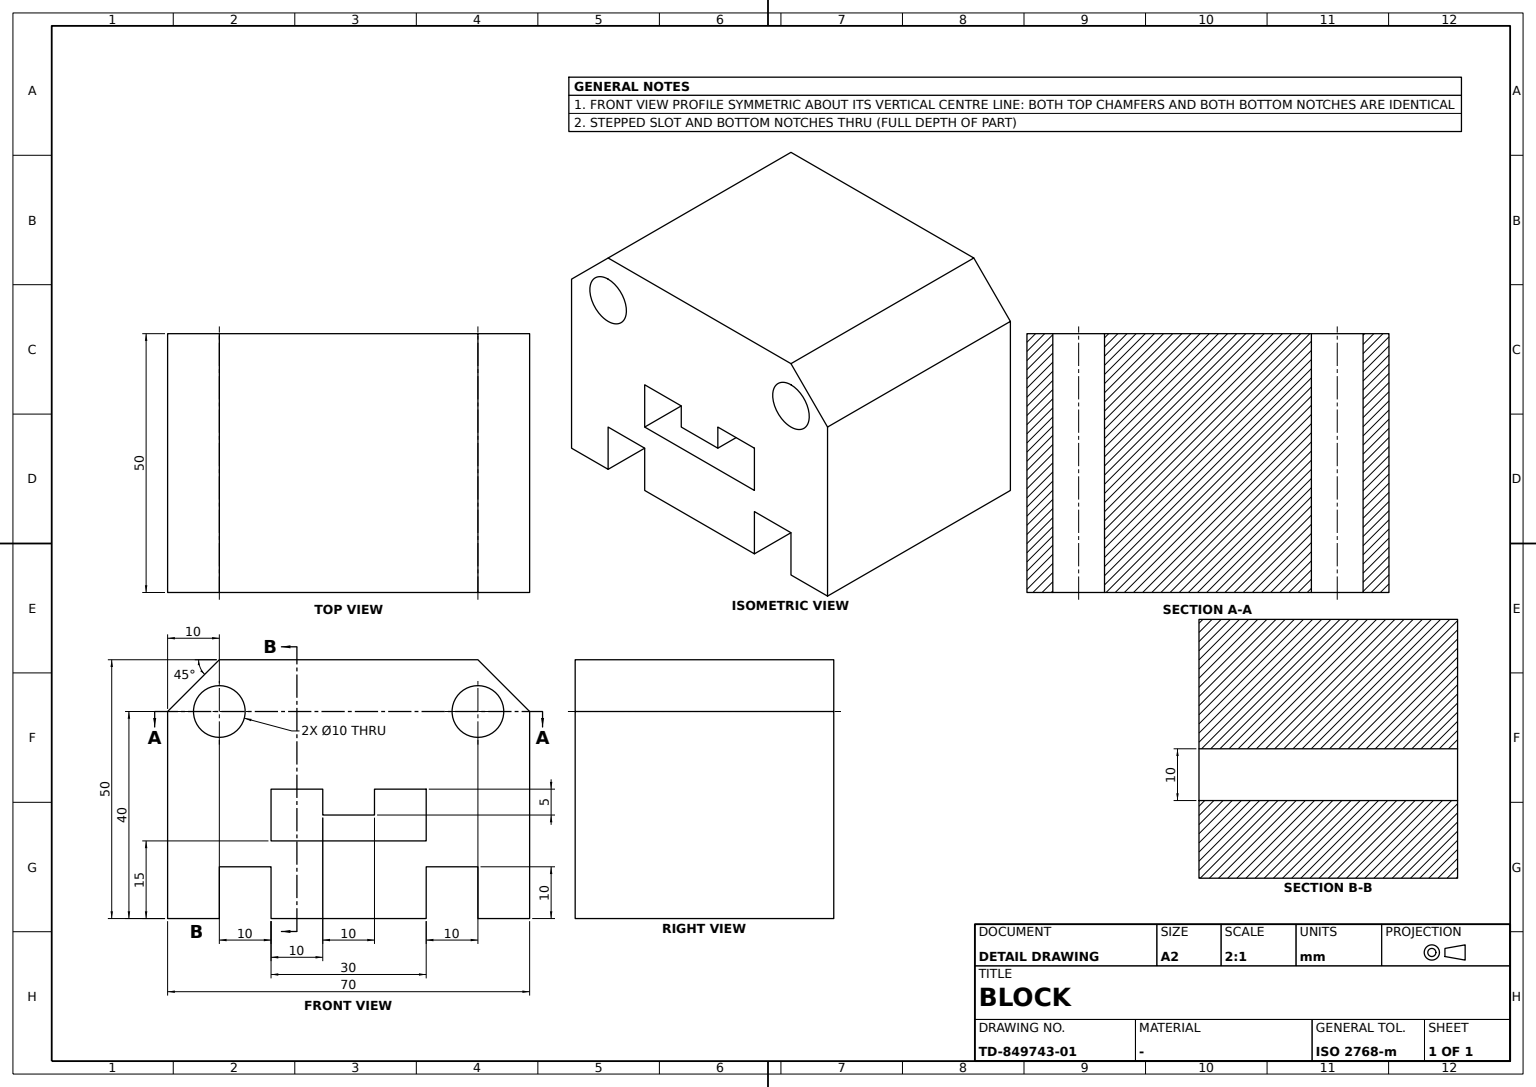
CATIA V5 part; units mm, degrees
sketch "Sketch1" plane through (0, 0, 0) normal (0, 0, 1) x (1, 0, 0)
  line L0 (-35, 25) -> (35, 25)
  line L1 (35, 25) -> (35, -25)
  line L2 (35, -25) -> (-35, -25)
  line L3 (-35, -25) -> (-35, 25)
  dimension "length L2" = 70
  dimension "length L3" = 50
  constraint horizontal L0 x-axis
  constraint horizontal L2 x-axis
  constraint vertical L1 y-axis
  constraint vertical L3 y-axis
  constraint symmetry L3 L1 y-axis
  constraint symmetry L0 L2 x-axis
extrude "Pad1" add sketch "Sketch1" along normal blind 50
sketch "Sketch2" plane through (0, 25, 0) normal (0, 1, 0) x (-1, 0, 0)
  line L0 (-35, 0) -> (35, 0) construction
  line L1 (-25, 0) -> (-15, 0)
  line L2 (15, 0) -> (25, 0)
  point P0 (-25, 0)
  line L3 (-25, 0) -> (-25, 10)
  line L4 (-25, 10) -> (-15, 10)
  line L5 (-15, 10) -> (-15, 0)
  point P1 (-15, 0)
  point P2 (15, 0)
  line L6 (15, 0) -> (15, 10)
  point P3 (15, 10)
  line L7 (15, 10) -> (25, 10)
  line L8 (25, 10) -> (25, 0)
  line L9 (-35, 0) -> (-35, 50) construction
  dimension "length L3" = 10
  dimension "length L4" = 10
  dimension "length L7" = 10
  dimension "distance L5 L6" = 30
  dimension "distance L9 L3" = 10
  constraint coincidence P0 L0
  constraint coincidence P1 L0
  constraint coincidence P2 L0
  constraint coincidence P3 L4
  constraint vertical L3 y-axis
  constraint vertical L5 y-axis
  constraint vertical L6 y-axis
  constraint vertical L8 y-axis
  constraint horizontal L4 x-axis
  constraint horizontal L7 x-axis
extrude "Pocket1" cut sketch "Sketch2" against normal through all
chamfer "Chamfer1" distance 10 angle 45 2 edges at (-35, 0, 50) (35, 0, 50)
sketch "Sketch3" plane through (0, 25, 0) normal (0, 1, 0) x (-1, 0, 0)
  line L0 (-15, 15) -> (15, 15)
  line L1 (15, 15) -> (15, 25)
  line L2 (15, 25) -> (5, 25)
  line L3 (5, 25) -> (5, 20)
  line L4 (5, 20) -> (-5, 20)
  line L5 (-5, 20) -> (-5, 25)
  point P0 (-5, 25)
  line L6 (-5, 25) -> (-15, 25)
  line L7 (-15, 25) -> (-15, 15)
  dimension "length L0" = 30
  dimension "length L2" = 10
  dimension "length L6" = 10
  dimension "distance L0 x axis" = 15
  dimension "length L7" = 10
  dimension "length L5" = 5
  constraint horizontal L0 x-axis
  constraint horizontal L2 x-axis
  constraint horizontal L4 x-axis
  constraint horizontal L6 x-axis
  constraint vertical L1 y-axis
  constraint vertical L3 y-axis
  constraint vertical L5 y-axis
  constraint vertical L7 y-axis
  constraint coincidence P0 L2
  constraint symmetry L7 L1 y-axis
extrude "Pocket2" cut sketch "Sketch3" against normal through all
sketch "Sketch4" plane through (0, 25, 0) normal (0, 1, 0) x (-1, 0, 0)
  circle A0 centre (25, 40) radius 5
  point P0 (25, 40)
  circle A1 centre (-25, 40) radius 5
  point P1 (-25, 40)
  line L0 (-35, 50) -> (35, 50) construction
  line L1 (-35, 50) -> (35, 50) construction
  line L2 (-35, 0) -> (-35, 50) construction
  line L3 (35, 0) -> (35, 50) construction
  dimension "radius A0" = 5
  dimension "radius A1" = 5
  dimension "distance P1 L0" = 10
  dimension "distance L1 P0" = 10
  dimension "distance L2 P1" = 10
  dimension "distance P0 L3" = 10
extrude "Pocket3" cut sketch "Sketch4" against normal through all
